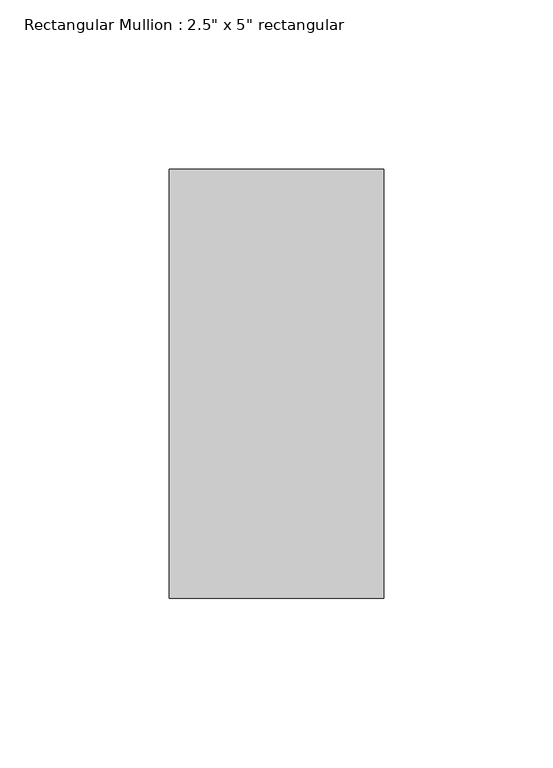
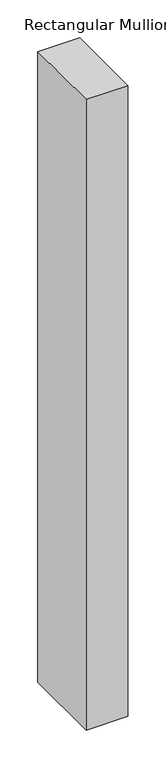
"""IFC4 building model written with IfcOpenShell, lengths in millimetres: member geometry."""

from ifc_helpers import new_model, si_unit, frame, origin, place, context, project, spatial, polyline, outline, extrude, source, transform, mapped, element, save


def member_f92b8aa2(model_context):
    return source(origin(), model_context, "Body", "SweptSolid", [
        extrude(outline(polyline([(31.75, 63.5), (31.75, -63.5), (-31.75, -63.5), (-31.75, 63.5), (31.75, 63.5)])), frame((0.0, 0.0, -1016.0), z_axis=(0.0, 0.0, 1.0), x_axis=(1.0, 0.0, 0.0)), (0.0, 0.0, 1.0), 1016.0),
    ])


if __name__ == "__main__":
    model = new_model("IFC4")
    model_context = context("Model", 3, world=origin())
    ifc_project = project(units=[si_unit("LENGTHUNIT", "METRE", prefix="MILLI")], contexts=[model_context])
    site = spatial("IfcSite", under=ifc_project)
    building = spatial("IfcBuilding", under=site)
    placement = place(None, origin())
    member_shape = member_f92b8aa2(model_context)
    element("IfcMember", 1, ObjectType="Rectangular Mullion : 2.5\" x 5\" rectangular", at=placement, inside=building, context=model_context, shape_type="MappedRepresentation", body=[
        mapped(member_shape, transform((0.0, 0.0, 0.0), x_axis=(1.0, 0.0, 0.0), y_axis=(0.0, 1.0, 0.0), z_axis=(0.0, 0.0, 1.0))),
    ])
    save(model, "model.ifc")

# Revit data of these elements
# Type "Rectangular Mullion : 2.5\" x 5\" rectangular"
#   built-in parameter 1007304 = 0.416667 (stored number, unit not read)
#   built-in parameter 1007301 = 0.104167 (stored number, unit not read)
#   built-in parameter 1007300 = 0.104167 (stored number, unit not read)
# Element 1 (IfcMember, "Rectangular Mullion : 2.5\" x 5\" rectangular")
#   Materials on its faces: "Aluminum"
# Materials
#   "Aluminum": class "Metal", colour RGB 247 247 247, transparency 0, Description = "Aluminum 6061", Cost = 0
